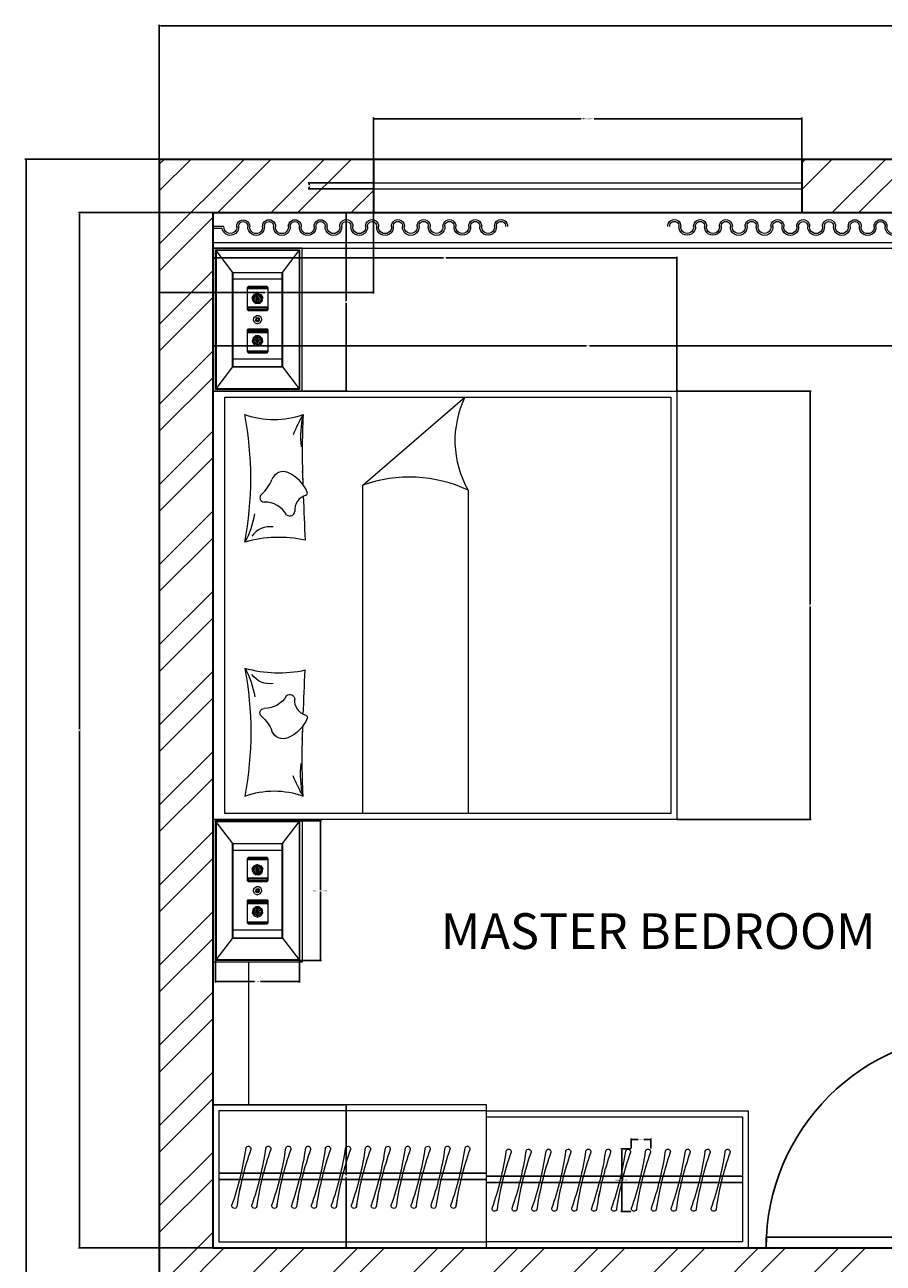
# Model space of a CAD drawing. Units: inches. Extents: x 3449 to 3843, y 1566 to 2054.
# Tile 6 of 8: x 3449 to 3594, y 1846 to 2054. Entities that reach past the tile are written whole.
import ezdxf

# ---------------------------------------------------------------- set-up
doc = ezdxf.new("R2010")
doc.units = ezdxf.units.IN
for name, color, linetype, lineweight in [('A-ANNO-DIMS', 2, 'Continuous', 18), ('A-AREA-IDEN', 7, 'Continuous', 25), ('A-DOOR', 4, 'Continuous', 25), ('A-FLOR-CASE', 7, 'Continuous', 20), ('A-FURN-DRAP', 32, 'Continuous', 13), ('A-GLAZ', 5, 'Continuous', 18), ('A-WALL', 7, 'Continuous', 35), ('A-WALL-PATT', 251, 'Continuous', 13), ('furn', 7, 'Continuous', 18)]:
    doc.layers.add(name, color=color, linetype=linetype, lineweight=lineweight)
doc.styles.get("Standard").update_dxf_attribs({"font": 'arial.ttf'})
doc.dimstyles.get("Standard").update_dxf_attribs({"dimtxt": 0.18, "dimasz": 0.18, "dimexe": 0.18, "dimexo": 0.0625, "dimgap": 0.09, "dimtad": 0, "dimtih": 1, "dimtoh": 1, "dimdec": 4, "dimzin": 0, "dimdsep": 46, "dimtxsty": 'Standard', "dimcen": 0.09, "dimadec": 0, "dimazin": 0, "dimtfac": 1, "dimtdec": 4, "dimtofl": 0, "dimtmove": 0, "dimatfit": 3, "dimfxl": 1, "dimtolj": 1, "dimtzin": 0, "dimarcsym": 0})

# ---------------------------------------------------------------- blocks, each defined once
blk = doc.blocks.new('*U5')
for p, q in [((0, 0), (0, -6)), ((36, 0), (36, -6))]:
    blk.add_line(p, q)
blk.add_lwpolyline([(0, 0), (0, 36), (1.75, 36), (1.75, 0)], close=True)
blk.add_arc((0, 0), 36, 0, 90)
blk = doc.blocks.new('12PLMP48')
for p, q in [((-4.94, 8.22), (-5, 8.31)), ((-5, 8.31), (5, 8.31)), ((-5, -8.31), (-5, 8.31)), ((-2.96, 5.62), (-4.94, 8.22)), ((4.94, 8.22), (-4.94, 8.22)), ((-4.94, 8.22), (-4.94, -8.22)), ((2.96, 5.62), (4.94, 8.22)), ((5, 8.31), (4.94, 8.22)), ((4.94, 8.22), (4.94, -8.22)), ((5, 8.31), (5, -8.31)), ((-2.94, 5.59), (-3, 5.62)), ((-3, 5.62), (3, 5.62)), ((-3, -5.63), (-3, 5.62)), ((2.94, 5.59), (-2.94, 5.59)), ((-2.94, 5.59), (-2.94, -5.59)), ((2.94, 4.81), (-2.94, 4.81)), ((3, 5.62), (2.94, 5.59)), ((2.94, -5.59), (2.94, 5.59)), ((3, -5.63), (3, 5.62)), ((-1.13, 3.94), (-1.25, 3.81)), ((-1.13, 3.84), (-1.25, 3.72)), ((-1.25, 3.81), (-1.25, 1.22)), ((-1.25, 3.72), (1.25, 3.72)), ((1.13, 3.94), (-1.13, 3.94)), ((-1.13, 3.84), (-1.13, 3.94)), ((1.13, 3.84), (-1.13, 3.84)), ((-0.62, 2.61), (-0.4, 2.98)), ((0, 3.12), (-0.4, 2.98)), ((-0.4, 2.98), (-0.32, 2.88)), ((0, 3), (-0.32, 2.88)), ((0, 2.5), (0, 3.12)), ((0, 3.12), (0.4, 2.98)), ((0.32, 2.88), (0, 3)), ((0.32, 2.88), (0.4, 2.98)), ((0.4, 2.98), (0.62, 2.61)), ((1.25, 3.81), (1.13, 3.94)), ((1.13, 3.84), (1.13, 3.94)), ((1.25, 3.72), (1.13, 3.84)), ((1.25, 1.22), (1.25, 3.81)), ((-1.13, 1.41), (-1.25, 1.53)), ((-1.25, 1.53), (1.25, 1.53)), ((0, 2.5), (-0.62, 2.61)), ((-0.54, 2.19), (-0.62, 2.61)), ((-0.38, 2.28), (-0.54, 2.19)), ((-0.54, 2.19), (-0.21, 1.91)), ((-0.32, 2.88), (-0.49, 2.59)), ((-0.49, 2.59), (-0.43, 2.25)), ((-0.43, 2.58), (-0.28, 2.83)), ((-0.38, 2.28), (-0.43, 2.58)), ((-0.43, 2.25), (-0.17, 2.03)), ((0, 2.5), (-0.38, 2.28)), ((-0.15, 2.09), (-0.38, 2.28)), ((-0.32, 2.88), (-0.32, 2.88)), ((-0.32, 2.88), (-0.28, 2.83)), ((-0.28, 2.83), (0, 2.94)), ((-0.28, 2.83), (0, 2.5)), ((-0.21, 1.91), (0, 2.5)), ((0.21, 1.91), (-0.21, 1.91)), ((-0.17, 2.03), (0.17, 2.03)), ((0.15, 2.09), (-0.15, 2.09)), ((-0.08, 2.6), (-0.12, 2.52)), ((-0.12, 2.52), (-0.11, 2.44)), ((-0.11, 2.44), (-0.04, 2.38)), ((0, 2.62), (-0.08, 2.6)), ((-0.04, 2.38), (0.04, 2.38)), ((0, 2.94), (0.28, 2.83)), ((0, 2.5), (0.32, 2.88)), ((0.08, 2.6), (0, 2.62)), ((0.62, 2.61), (0, 2.5)), ((0.54, 2.19), (0, 2.5)), ((0, 2.5), (0.21, 1.91)), ((0.04, 2.38), (0.11, 2.44)), ((0.12, 2.52), (0.08, 2.6)), ((0.11, 2.44), (0.12, 2.52)), ((0.38, 2.28), (0.15, 2.09)), ((0.17, 2.03), (0.43, 2.25)), ((0.21, 1.91), (0.54, 2.19)), ((0.28, 2.83), (0.43, 2.58)), ((0.49, 2.59), (0.32, 2.88)), ((0.32, 2.88), (0.32, 2.88)), ((0.43, 2.58), (0.38, 2.28)), ((0.43, 2.25), (0.49, 2.59)), ((0.54, 2.19), (0.62, 2.61)), ((1.25, 1.53), (1.13, 1.41)), ((-1.13, 1.25), (-1.25, 1.37)), ((-1.25, 1.22), (-1.13, 1.09)), ((1.13, 1.41), (-1.13, 1.41)), ((-1.13, 1.41), (-1.13, 1.09)), ((-1.13, 1.25), (1.13, 1.25)), ((-1.13, 1.09), (1.13, 1.09)), ((-0.49, -0.09), (-0.43, 0.25)), ((-0.43, 0.25), (-0.17, 0.47)), ((-0.22, 0.12), (-0.25, -0.04)), ((-0.09, 0.23), (-0.22, 0.12)), ((0.17, 0.47), (-0.17, 0.47)), ((-0.12, -0.12), (-0.12, 0.12)), ((-0.12, 0.12), (0.12, 0.12)), ((-0.09, 0.23), (0.09, 0.23)), ((0.22, 0.12), (0.09, 0.23)), ((0.12, 0.12), (0.12, -0.12)), ((0.43, 0.25), (0.17, 0.47)), ((0.25, -0.04), (0.22, 0.12)), ((0.43, 0.25), (0.49, -0.09)), ((1.13, 1.09), (1.13, 1.41)), ((1.13, 1.25), (1.25, 1.37)), ((1.13, 1.09), (1.25, 1.22)), ((-1.25, -1.22), (-1.13, -1.09)), ((-1.25, -1.22), (-1.25, -3.81)), ((-1.13, -1.25), (-1.25, -1.38)), ((-1.13, -1.41), (-1.25, -1.53)), ((-1.13, -1.41), (-1.13, -1.09)), ((-1.13, -1.09), (1.13, -1.09)), ((1.13, -1.25), (-1.13, -1.25)), ((1.13, -1.41), (-1.13, -1.41)), ((-0.32, -0.38), (-0.49, -0.09)), ((-0.32, -0.38), (0, -0.5)), ((-0.16, -0.19), (-0.25, -0.04)), ((0, -0.25), (-0.16, -0.19)), ((0.12, -0.12), (-0.12, -0.12)), ((0.16, -0.19), (0, -0.25)), ((0.32, -0.38), (0, -0.5)), ((0.16, -0.19), (0.25, -0.04)), ((0.32, -0.38), (0.49, -0.09)), ((1.13, -1.41), (1.13, -1.09)), ((1.13, -1.09), (1.25, -1.22)), ((1.25, -1.38), (1.13, -1.25)), ((1.25, -1.53), (1.13, -1.41)), ((1.25, -3.81), (1.25, -1.22)), ((-1.25, -1.53), (1.25, -1.53)), ((-0.54, -2.19), (-0.62, -2.61)), ((0, -2.5), (-0.62, -2.61)), ((-0.62, -2.61), (-0.4, -2.98)), ((-0.21, -1.91), (-0.54, -2.19)), ((-0.54, -2.19), (0, -2.5)), ((-0.49, -2.59), (-0.43, -2.25)), ((-0.32, -2.88), (-0.49, -2.59)), ((-0.43, -2.25), (-0.17, -2.03)), ((-0.43, -2.58), (-0.38, -2.28)), ((-0.28, -2.84), (-0.43, -2.58)), ((-0.4, -2.98), (-0.32, -2.88)), ((-0.38, -2.28), (-0.15, -2.09)), ((-0.32, -2.88), (-0.28, -2.84)), ((0, -3), (-0.32, -2.88)), ((-0.28, -2.84), (-0.08, -2.6)), ((0, -2.94), (-0.28, -2.84)), ((0.21, -1.91), (-0.21, -1.91)), ((0, -2.5), (-0.21, -1.91)), ((-0.17, -2.03), (0.17, -2.03)), ((-0.15, -2.09), (0.15, -2.09)), ((-0.11, -2.44), (-0.12, -2.52)), ((-0.12, -2.52), (-0.08, -2.6)), ((-0.04, -2.38), (-0.11, -2.44)), ((-0.08, -2.6), (0, -2.5)), ((-0.08, -2.6), (0, -2.63)), ((0.04, -2.38), (-0.04, -2.38)), ((0, -2.5), (0.21, -1.91)), ((0.11, -2.44), (0, -2.5)), ((0, -3.13), (0, -2.5)), ((0, -2.5), (0.4, -2.98)), ((0.62, -2.61), (0, -2.5)), ((0, -2.63), (0.08, -2.6)), ((0.28, -2.84), (0, -2.94)), ((0.32, -2.88), (0, -3)), ((0.11, -2.44), (0.04, -2.38)), ((0.08, -2.6), (0.12, -2.52)), ((0.38, -2.28), (0.11, -2.44)), ((0.12, -2.52), (0.11, -2.44)), ((0.15, -2.09), (0.38, -2.28)), ((0.17, -2.03), (0.43, -2.25)), ((0.21, -1.91), (0.54, -2.19)), ((0.43, -2.58), (0.28, -2.84)), ((0.49, -2.59), (0.32, -2.88)), ((0.54, -2.19), (0.38, -2.28)), ((0.38, -2.28), (0.43, -2.58)), ((0.4, -2.98), (0.62, -2.61)), ((0.43, -2.25), (0.49, -2.59)), ((0.62, -2.61), (0.54, -2.19)), ((-1.13, -3.84), (-1.25, -3.72)), ((-1.25, -3.72), (1.25, -3.72)), ((-1.25, -3.81), (-1.13, -3.94)), ((-1.13, -3.94), (-1.13, -3.84)), ((1.13, -3.84), (-1.13, -3.84)), ((-1.13, -3.94), (1.13, -3.94)), ((-0.4, -2.98), (0, -3.13)), ((0, -3.13), (0.4, -2.98)), ((1.25, -3.72), (1.13, -3.84)), ((1.13, -3.94), (1.25, -3.81)), ((1.13, -3.94), (1.13, -3.84)), ((-4.94, -8.22), (-2.96, -5.63)), ((-2.94, -5.59), (-3, -5.63)), ((-3, -5.63), (3, -5.63)), ((2.94, -4.69), (-2.94, -4.69)), ((-2.94, -5.59), (2.94, -5.59)), ((3, -5.63), (2.94, -5.59)), ((2.96, -5.63), (4.94, -8.22)), ((-4.94, -8.22), (-5, -8.31)), ((5, -8.31), (-5, -8.31)), ((4.94, -8.22), (-4.94, -8.22)), ((4.94, -8.22), (5, -8.31))]:
    blk.add_line(p, q)
blk = doc.blocks.new('PILLOW-BED')
for centre, radius, start, end in [((-58.04, 10.73), 59.02, 349.525, 10.475), ((4.89, 35.06), 14.45, 250.2291, 289.7709), ((27.88, 10.54), 21.14, 148.9025, 159.1397), ((25.99, 17.7), 16.64, 166.9326, 185.8487), ((149.01, 15.02), 139.38, 177.3527, 182.1874), ((370.18, 15.14), 360.55, 180.0403, 180.0472), ((-1.15, 12.67), 6.07, 310.2522, 339.5725), ((6.42, 9.85), 2, 66.6818, 159.5725), ((4.74, 5.96), 6.24, 23.0209, 66.6818), ((56.2, 13.08), 46.57, 181.419, 184.1998), ((10.15, 8.25), 0.362, 287.5153, 24.7447), ((3.25, 7.48), 0.73, 130.2522, 270.4936), ((3.29, 2.5), 4.25, 29.3034, 90.4936), ((10.95, 5.41), 2.59, 105.4046, 185.5925), ((370.18, 19.17), 360.55, 181.8172, 182.9967), ((-12.31, 6.94), 14.13, 330.5975, 351.1793), ((7.53, 5.25), 0.85, 231.2945, 354.0462), ((4.17, -1.03), 3.63, 80.7217, 145.7354), ((5.68, -19.42), 20.23, 77.3054, 106.2929)]:
    blk.add_arc(centre, radius, start, end)
blk = doc.blocks.new('DRAPERY-PANEL')
for p, q in [((1.19, 47.95), (1.19, 49.52)), ((1.5, 47.66), (1.5, 49.52))]:
    blk.add_line(p, q)
for centre, radius, start, end in [((1.42, 46.57), 1.4, 99.481, 274.2422), ((1.42, 46.57), 1.09, 85.7578, 274.2422), ((1.55, 44.41), 1.09, 265.7578, 94.2422), ((1.55, 44.41), 0.776, 265.7578, 94.2422), ((1.4, 42.24), 1.4, 85.7578, 274.2422), ((1.4, 42.24), 1.09, 85.7578, 274.2422), ((1.56, 40.07), 1.09, 265.7578, 94.2422), ((1.56, 40.07), 0.776, 265.7578, 94.2422), ((1.4, 37.91), 1.4, 85.7578, 274.2422), ((1.4, 37.91), 1.09, 85.7578, 274.2422), ((1.56, 35.74), 1.09, 265.7578, 94.2422), ((1.56, 35.74), 0.776, 265.7578, 94.2422), ((1.4, 33.58), 1.4, 85.7578, 274.2422), ((1.4, 33.58), 1.09, 85.7578, 274.2422), ((1.56, 31.41), 1.09, 265.7578, 94.2422), ((1.56, 31.41), 0.776, 265.7578, 94.2422), ((1.41, 29.24), 1.4, 85.7578, 274.2422), ((1.41, 29.24), 1.09, 85.7578, 274.2422), ((1.57, 27.08), 1.09, 265.7578, 94.2422), ((1.57, 27.08), 0.776, 265.7578, 94.2422), ((1.41, 24.91), 1.4, 85.7578, 274.2422), ((1.41, 24.91), 1.09, 85.7578, 274.2422), ((1.57, 22.74), 1.09, 265.7578, 94.2422), ((1.57, 22.74), 0.776, 265.7578, 94.2422), ((1.41, 20.58), 1.4, 85.7578, 274.2422), ((1.41, 20.58), 1.09, 85.7578, 274.2422), ((1.58, 18.41), 1.09, 265.7578, 94.2422), ((1.58, 18.41), 0.776, 265.7578, 94.2422), ((1.42, 16.25), 1.4, 85.7578, 274.2422), ((1.42, 16.25), 1.09, 85.7578, 274.2422), ((1.58, 14.08), 1.09, 265.7578, 94.2422), ((1.58, 14.08), 0.776, 265.7578, 94.2422), ((1.42, 11.91), 1.4, 85.7578, 274.2422), ((1.42, 11.91), 1.09, 85.7578, 274.2422), ((1.58, 9.75), 1.09, 265.7578, 94.2422), ((1.58, 9.75), 0.776, 265.7578, 94.2422), ((1.43, 7.58), 1.4, 85.7578, 274.2422), ((1.43, 7.58), 1.09, 85.7578, 274.2422), ((1.59, 5.42), 1.09, 265.7578, 94.2422), ((1.43, 3.25), 1.4, 85.7578, 274.2422), ((1.43, 3.25), 1.09, 85.7578, 274.2422), ((1.59, 5.42), 0.776, 265.7578, 94.2422), ((1.59, 1.08), 1.09, 265.7578, 94.2422), ((1.59, 1.08), 0.776, 265.7578, 94.2422)]:
    blk.add_arc(centre, radius, start, end)
blk = doc.blocks.new('DRAPERY-PANEL-CAPPED')
for p, q in [((1.19, 1.57), (1.19, 0)), ((1.19, 0), (1.5, 0)), ((1.5, 1.86), (1.5, 0))]:
    blk.add_line(p, q)
for centre, radius, start, end in [((1.59, 48.44), 1.09, 265.7578, 94.2422), ((1.59, 48.44), 0.776, 265.7578, 94.2422), ((1.43, 46.27), 1.4, 85.7578, 274.2422), ((1.43, 46.27), 1.09, 85.7578, 274.2422), ((1.59, 44.1), 1.09, 265.7578, 94.2422), ((1.59, 44.1), 0.776, 265.7578, 94.2422), ((1.43, 41.94), 1.4, 85.7578, 274.2422), ((1.43, 41.94), 1.09, 85.7578, 274.2422), ((1.58, 39.77), 1.09, 265.7578, 94.2422), ((1.58, 39.77), 0.776, 265.7578, 94.2422), ((1.42, 37.6), 1.4, 85.7578, 274.2422), ((1.42, 37.6), 1.09, 85.7578, 274.2422), ((1.58, 35.44), 1.09, 265.7578, 94.2422), ((1.58, 35.44), 0.776, 265.7578, 94.2422), ((1.42, 33.27), 1.4, 85.7578, 274.2422), ((1.42, 33.27), 1.09, 85.7578, 274.2422), ((1.58, 31.11), 1.09, 265.7578, 94.2422), ((1.58, 31.11), 0.776, 265.7578, 94.2422), ((1.41, 28.94), 1.4, 85.7578, 274.2422), ((1.41, 28.94), 1.09, 85.7578, 274.2422), ((1.57, 26.77), 1.09, 265.7578, 94.2422), ((1.57, 26.77), 0.776, 265.7578, 94.2422), ((1.41, 24.61), 1.4, 85.7578, 274.2422), ((1.41, 24.61), 1.09, 85.7578, 274.2422), ((1.57, 22.44), 1.09, 265.7578, 94.2422), ((1.57, 22.44), 0.776, 265.7578, 94.2422), ((1.41, 20.28), 1.4, 85.7578, 274.2422), ((1.41, 20.28), 1.09, 85.7578, 274.2422), ((1.56, 18.11), 1.09, 265.7578, 94.2422), ((1.56, 18.11), 0.776, 265.7578, 94.2422), ((1.4, 15.94), 1.4, 85.7578, 274.2422), ((1.4, 15.94), 1.09, 85.7578, 274.2422), ((1.56, 13.78), 1.09, 265.7578, 94.2422), ((1.4, 11.61), 1.4, 85.7578, 274.2422), ((1.4, 11.61), 1.09, 85.7578, 274.2422), ((1.56, 13.78), 0.776, 265.7578, 94.2422), ((1.56, 9.45), 1.09, 265.7578, 94.2422), ((1.4, 7.28), 1.4, 85.7578, 274.2422), ((1.4, 7.28), 1.09, 85.7578, 274.2422), ((1.56, 9.45), 0.776, 265.7578, 94.2422), ((1.42, 2.95), 1.4, 85.7578, 260.519), ((1.55, 5.11), 1.09, 265.7578, 94.2422), ((1.55, 5.11), 0.776, 265.7578, 94.2422), ((1.42, 2.95), 1.09, 85.7578, 274.2422)]:
    blk.add_arc(centre, radius, start, end)
blk = doc.blocks.new('WARDROBE-HANGER-A')
at = {"transparency": 33554687}
blk.add_lwpolyline([(2.38, 10.13, -1), (3.19, 9.92, 0.050016), (0.83, 0.32, -1), (0.01, 0.52, 0.050016)], format="xyb", close=True, dxfattribs=at)
blk.add_arc((49.86, -6.67), 49.53, 160.4279, 171.8811, dxfattribs=at)
blk = doc.blocks.new('WARDROBE-HANGER-B')
at = {"transparency": 33554687}
blk.add_lwpolyline([(2.37, 10.13, -1), (3.19, 9.92, 0.050016), (0.83, 0.32, -1), (0.01, 0.52, 0.050016)], format="xyb", close=True, dxfattribs=at)
blk.add_arc((49.86, -6.67), 49.53, 160.4279, 171.8811, dxfattribs=at)
blk = doc.blocks.new('GLAZING-72')
for p, q in [((0, 1), (72, 1)), ((0, 0), (72, 0))]:
    blk.add_line(p, q)
blk = doc.blocks.new('*D36')
at = {"layer": 'A-ANNO-DIMS', "color": 0, "lineweight": -2, "transparency": 16777216}
for p, q in [((3551.34, 1865.22), (3549.65, 1865.22)), ((3549.83, 1865.04), (3549.83, 1860.14)), ((3549.83, 1854.87), (3549.83, 1859.77)), ((3551.34, 1854.69), (3549.65, 1854.69))]:
    blk.add_line(p, q, dxfattribs=at)
at = {"layer": 'A-ANNO-DIMS', "color": 0, "transparency": 16777216}
for points in [[(3549.8, 1865.04), (3549.86, 1865.04), (3549.83, 1865.22)], [(3549.8, 1854.87), (3549.86, 1854.87), (3549.83, 1854.69)]]:
    blk.add_solid(points, dxfattribs=at)
at = {"layer": 'Defpoints', "color": 0, "transparency": 16777216}
for p in [(3549.83, 1865.22), (3551.41, 1865.22), (3551.41, 1854.69)]:
    blk.add_point(p, dxfattribs=at)
at = {"layer": 'A-ANNO-DIMS', "color": 0, "transparency": 16777216, "insert": (3549.83, 1859.96), "char_height": 0.18, "attachment_point": 5}
blk.add_mtext('\\A1;HANGER B 11 TYP.', dxfattribs=at)
blk = doc.blocks.new('*D37')
at = {"layer": 'A-ANNO-DIMS', "color": 0, "lineweight": -2, "transparency": 16777216}
for p, q in [((3551.41, 1865.29), (3551.41, 1866.99)), ((3551.59, 1866.81), (3552.6, 1866.81)), ((3554.52, 1866.81), (3553.51, 1866.81)), ((3554.7, 1865.29), (3554.7, 1866.99))]:
    blk.add_line(p, q, dxfattribs=at)
at = {"layer": 'A-ANNO-DIMS', "color": 0, "transparency": 16777216}
for points in [[(3551.59, 1866.84), (3551.59, 1866.78), (3551.41, 1866.81)], [(3554.52, 1866.84), (3554.52, 1866.78), (3554.7, 1866.81)]]:
    blk.add_solid(points, dxfattribs=at)
at = {"layer": 'Defpoints', "color": 0, "transparency": 16777216}
for p in [(3554.7, 1866.81), (3551.41, 1865.22), (3554.7, 1865.22)]:
    blk.add_point(p, dxfattribs=at)
at = {"layer": 'A-ANNO-DIMS', "color": 0, "transparency": 16777216, "insert": (3553.05, 1866.81), "char_height": 0.18, "attachment_point": 5}
blk.add_mtext('\\A1;3 TYP.', dxfattribs=at)
blk = doc.blocks.new('*D44')
at = {"layer": 'A-ANNO-DIMS', "color": 0, "lineweight": -2, "transparency": 16777216}
for p, q in [((3495.73, 1920.36), (3499.36, 1920.36)), ((3499.18, 1920.18), (3499.18, 1908.8)), ((3499.18, 1897.07), (3499.18, 1908.44)), ((3495.73, 1896.89), (3499.36, 1896.89))]:
    blk.add_line(p, q, dxfattribs=at)
at = {"layer": 'A-ANNO-DIMS', "color": 0, "transparency": 16777216}
for points in [[(3499.15, 1920.18), (3499.21, 1920.18), (3499.18, 1920.36)], [(3499.15, 1897.07), (3499.21, 1897.07), (3499.18, 1896.89)]]:
    blk.add_solid(points, dxfattribs=at)
at = {"layer": 'Defpoints', "color": 0, "transparency": 16777216}
for p in [(3495.66, 1920.36), (3499.18, 1920.36), (3495.66, 1896.89)]:
    blk.add_point(p, dxfattribs=at)
at = {"layer": 'A-ANNO-DIMS', "color": 0, "transparency": 16777216, "insert": (3499.18, 1908.62), "char_height": 0.18, "attachment_point": 5}
blk.add_mtext('\\A1;NIGHTSTAND 23 TYP.', dxfattribs=at)
blk = doc.blocks.new('*D45')
at = {"layer": 'A-ANNO-DIMS', "color": 0, "lineweight": -2, "transparency": 16777216}
for p, q in [((3481.55, 1896.82), (3481.55, 1893.18)), ((3495.66, 1896.82), (3495.66, 1893.18)), ((3481.73, 1893.36), (3488.09, 1893.36)), ((3495.48, 1893.36), (3489.12, 1893.36))]:
    blk.add_line(p, q, dxfattribs=at)
at = {"layer": 'A-ANNO-DIMS', "color": 0, "transparency": 16777216}
for points in [[(3481.73, 1893.39), (3481.73, 1893.33), (3481.55, 1893.36)], [(3495.48, 1893.39), (3495.48, 1893.33), (3495.66, 1893.36)]]:
    blk.add_solid(points, dxfattribs=at)
at = {"layer": 'Defpoints', "color": 0, "transparency": 16777216}
for p in [(3481.55, 1896.89), (3495.66, 1896.89), (3495.66, 1893.36)]:
    blk.add_point(p, dxfattribs=at)
at = {"layer": 'A-ANNO-DIMS', "color": 0, "transparency": 16777216, "insert": (3488.6, 1893.36), "char_height": 0.18, "attachment_point": 5}
blk.add_mtext('\\A1;14 TYP.', dxfattribs=at)
blk = doc.blocks.new('*D60')
at = {"layer": 'A-ANNO-DIMS', "color": 0, "lineweight": -2, "transparency": 16777216}
for p, q in [((3508.09, 2027.68), (3508.09, 2038.59)), ((3508.27, 2038.41), (3542.97, 2038.41)), ((3579.91, 2038.41), (3545.21, 2038.41)), ((3580.09, 2027.68), (3580.09, 2038.59))]:
    blk.add_line(p, q, dxfattribs=at)
at = {"layer": 'A-ANNO-DIMS', "color": 0, "transparency": 16777216}
for points in [[(3508.27, 2038.44), (3508.27, 2038.38), (3508.09, 2038.41)], [(3579.91, 2038.44), (3579.91, 2038.38), (3580.09, 2038.41)]]:
    blk.add_solid(points, dxfattribs=at)
at = {"layer": 'Defpoints', "color": 0, "transparency": 16777216}
for p in [(3580.09, 2038.41), (3508.09, 2027.61), (3580.09, 2027.61)]:
    blk.add_point(p, dxfattribs=at)
at = {"layer": 'A-ANNO-DIMS', "color": 0, "transparency": 16777216, "insert": (3544.09, 2038.41), "char_height": 0.18, "attachment_point": 5}
blk.add_mtext('\\A1;WINDOW 72 TYP.', dxfattribs=at)
blk = doc.blocks.new('*D61')
at = {"layer": 'A-ANNO-DIMS', "color": 0, "lineweight": -2, "transparency": 16777216}
for p, q in [((3508.03, 2027.61), (3497.11, 2027.61)), ((3508.03, 2026.61), (3497.11, 2026.61)), ((3497.29, 2027.43), (3497.29, 2027.29)), ((3497.29, 2026.79), (3497.29, 2026.93))]:
    blk.add_line(p, q, dxfattribs=at)
at = {"layer": 'A-ANNO-DIMS', "color": 0, "transparency": 16777216}
for points in [[(3497.26, 2027.43), (3497.32, 2027.43), (3497.29, 2027.61)], [(3497.26, 2026.79), (3497.32, 2026.79), (3497.29, 2026.61)]]:
    blk.add_solid(points, dxfattribs=at)
at = {"layer": 'Defpoints', "color": 0, "transparency": 16777216}
for p in [(3497.29, 2027.61), (3508.09, 2027.61), (3508.09, 2026.61)]:
    blk.add_point(p, dxfattribs=at)
at = {"layer": 'A-ANNO-DIMS', "color": 0, "transparency": 16777216, "insert": (3497.29, 2027.11), "char_height": 0.18, "attachment_point": 5}
blk.add_mtext('\\A1;1 TYP.', dxfattribs=at)
blk = doc.blocks.new('*D76')
at = {"layer": 'A-ANNO-DIMS', "color": 0, "lineweight": -2, "transparency": 16777216}
for p, q in [((3472.09, 2031.68), (3472.09, 2054.19)), ((3472.27, 2054.01), (3645.8, 2054.01)), ((3819.91, 2054.01), (3646.38, 2054.01)), ((3820.09, 1986.68), (3820.09, 2054.19))]:
    blk.add_line(p, q, dxfattribs=at)
at = {"layer": 'A-ANNO-DIMS', "color": 0, "transparency": 16777216}
for points in [[(3472.27, 2054.04), (3472.27, 2053.98), (3472.09, 2054.01)], [(3819.91, 2054.04), (3819.91, 2053.98), (3820.09, 2054.01)]]:
    blk.add_solid(points, dxfattribs=at)
at = {"layer": 'Defpoints', "color": 0, "transparency": 16777216}
for p in [(3820.09, 2054.01), (3472.09, 2031.61), (3820.09, 1986.61)]:
    blk.add_point(p, dxfattribs=at)
at = {"layer": 'A-ANNO-DIMS', "color": 0, "transparency": 16777216, "insert": (3646.09, 2054.01), "char_height": 0.18, "attachment_point": 5}
blk.add_mtext('\\A1;348', dxfattribs=at)
blk = doc.blocks.new('*D77')
at = {"layer": 'A-ANNO-DIMS', "color": 0, "lineweight": -2, "transparency": 16777216}
for p, q in [((3472.03, 2031.61), (3449.51, 2031.61)), ((3449.69, 2031.43), (3449.69, 1810.3)), ((3449.69, 1588.79), (3449.69, 1809.93)), ((3481.03, 1588.61), (3449.51, 1588.61))]:
    blk.add_line(p, q, dxfattribs=at)
at = {"layer": 'A-ANNO-DIMS', "color": 0, "transparency": 16777216}
for points in [[(3449.66, 2031.43), (3449.72, 2031.43), (3449.69, 2031.61)], [(3449.66, 1588.79), (3449.72, 1588.79), (3449.69, 1588.61)]]:
    blk.add_solid(points, dxfattribs=at)
at = {"layer": 'Defpoints', "color": 0, "transparency": 16777216}
for p in [(3449.69, 2031.61), (3472.09, 2031.61), (3481.09, 1588.61)]:
    blk.add_point(p, dxfattribs=at)
at = {"layer": 'A-ANNO-DIMS', "color": 0, "transparency": 16777216, "insert": (3449.69, 1810.11), "char_height": 0.18, "attachment_point": 5}
blk.add_mtext('\\A1;443', dxfattribs=at)
blk = doc.blocks.new('*D80')
at = {"layer": 'A-ANNO-DIMS', "color": 0, "lineweight": -2, "transparency": 16777216}
for p, q in [((3472.09, 2031.55), (3472.09, 2009.03)), ((3508.09, 2031.55), (3508.09, 2009.03)), ((3472.27, 2009.21), (3489.87, 2009.21)), ((3507.91, 2009.21), (3490.31, 2009.21))]:
    blk.add_line(p, q, dxfattribs=at)
at = {"layer": 'A-ANNO-DIMS', "color": 0, "transparency": 16777216}
for points in [[(3472.27, 2009.24), (3472.27, 2009.18), (3472.09, 2009.21)], [(3507.91, 2009.24), (3507.91, 2009.18), (3508.09, 2009.21)]]:
    blk.add_solid(points, dxfattribs=at)
at = {"layer": 'Defpoints', "color": 0, "transparency": 16777216}
for p in [(3472.09, 2031.61), (3508.09, 2031.61), (3472.09, 2009.21)]:
    blk.add_point(p, dxfattribs=at)
at = {"layer": 'A-ANNO-DIMS', "color": 0, "transparency": 16777216, "insert": (3490.09, 2009.21), "char_height": 0.18, "attachment_point": 5}
blk.add_mtext('\\A1;36', dxfattribs=at)
blk = doc.blocks.new('*D81')
at = {"layer": 'A-ANNO-DIMS', "color": 0, "lineweight": -2, "transparency": 16777216}
for p, q in [((3481.03, 2022.61), (3458.51, 2022.61)), ((3458.69, 2022.43), (3458.69, 1935.79)), ((3458.69, 1848.79), (3458.69, 1935.43)), ((3481.03, 1848.61), (3458.51, 1848.61))]:
    blk.add_line(p, q, dxfattribs=at)
at = {"layer": 'A-ANNO-DIMS', "color": 0, "transparency": 16777216}
for points in [[(3458.66, 2022.43), (3458.72, 2022.43), (3458.69, 2022.61)], [(3458.66, 1848.79), (3458.72, 1848.79), (3458.69, 1848.61)]]:
    blk.add_solid(points, dxfattribs=at)
at = {"layer": 'Defpoints', "color": 0, "transparency": 16777216}
for p in [(3458.69, 2022.61), (3481.09, 2022.61), (3481.09, 1848.61)]:
    blk.add_point(p, dxfattribs=at)
at = {"layer": 'A-ANNO-DIMS', "color": 0, "transparency": 16777216, "insert": (3458.69, 1935.61), "char_height": 0.18, "attachment_point": 5}
blk.add_mtext('\\A1;174', dxfattribs=at)
blk = doc.blocks.new('*D82')
at = {"layer": 'A-ANNO-DIMS', "color": 0, "lineweight": -2, "transparency": 16777216}
for p, q in [((3481.09, 2022.55), (3481.09, 2000.03)), ((3607.09, 2022.55), (3607.09, 2000.03)), ((3481.27, 2000.21), (3543.81, 2000.21)), ((3606.91, 2000.21), (3544.37, 2000.21))]:
    blk.add_line(p, q, dxfattribs=at)
at = {"layer": 'A-ANNO-DIMS', "color": 0, "transparency": 16777216}
for points in [[(3481.27, 2000.24), (3481.27, 2000.18), (3481.09, 2000.21)], [(3606.91, 2000.24), (3606.91, 2000.18), (3607.09, 2000.21)]]:
    blk.add_solid(points, dxfattribs=at)
at = {"layer": 'Defpoints', "color": 0, "transparency": 16777216}
for p in [(3481.09, 2022.61), (3607.09, 2022.61), (3481.09, 2000.21)]:
    blk.add_point(p, dxfattribs=at)
at = {"layer": 'A-ANNO-DIMS', "color": 0, "transparency": 16777216, "insert": (3544.09, 2000.21), "char_height": 0.18, "attachment_point": 5}
blk.add_mtext('\\A1;126', dxfattribs=at)
blk = doc.blocks.new('*D103')
at = {"layer": 'A-ANNO-DIMS', "color": 0, "lineweight": -2, "transparency": 16777216}
for p, q in [((3481.09, 1992.68), (3481.09, 2015.19)), ((3481.27, 2015.01), (3519.87, 2015.01)), ((3558.91, 2015.01), (3520.31, 2015.01)), ((3559.09, 1992.68), (3559.09, 2015.19))]:
    blk.add_line(p, q, dxfattribs=at)
at = {"layer": 'A-ANNO-DIMS', "color": 0, "transparency": 16777216}
for points in [[(3481.27, 2015.04), (3481.27, 2014.98), (3481.09, 2015.01)], [(3558.91, 2015.04), (3558.91, 2014.98), (3559.09, 2015.01)]]:
    blk.add_solid(points, dxfattribs=at)
at = {"layer": 'Defpoints', "color": 0, "transparency": 16777216}
for p in [(3559.09, 2015.01), (3481.09, 1992.61), (3559.09, 1992.61)]:
    blk.add_point(p, dxfattribs=at)
at = {"layer": 'A-ANNO-DIMS', "color": 0, "transparency": 16777216, "insert": (3520.09, 2015.01), "char_height": 0.18, "attachment_point": 5}
blk.add_mtext('\\A1;78', dxfattribs=at)
blk = doc.blocks.new('*D104')
at = {"layer": 'A-ANNO-DIMS', "color": 0, "lineweight": -2, "transparency": 16777216}
for p, q in [((3559.15, 1992.61), (3581.67, 1992.61)), ((3581.49, 1992.43), (3581.49, 1956.79)), ((3581.49, 1920.79), (3581.49, 1956.43)), ((3559.15, 1920.61), (3581.67, 1920.61))]:
    blk.add_line(p, q, dxfattribs=at)
at = {"layer": 'A-ANNO-DIMS', "color": 0, "transparency": 16777216}
for points in [[(3581.46, 1992.43), (3581.52, 1992.43), (3581.49, 1992.61)], [(3581.46, 1920.79), (3581.52, 1920.79), (3581.49, 1920.61)]]:
    blk.add_solid(points, dxfattribs=at)
at = {"layer": 'Defpoints', "color": 0, "transparency": 16777216}
for p in [(3559.09, 1992.61), (3559.09, 1920.61), (3581.49, 1920.61)]:
    blk.add_point(p, dxfattribs=at)
at = {"layer": 'A-ANNO-DIMS', "color": 0, "transparency": 16777216, "insert": (3581.49, 1956.61), "char_height": 0.18, "attachment_point": 5}
blk.add_mtext('\\A1;72', dxfattribs=at)
blk = doc.blocks.new('*D116')
at = {"layer": 'A-ANNO-DIMS', "color": 0, "lineweight": -2, "transparency": 16777216}
for p, q in [((3481.15, 2022.61), (3503.67, 2022.61)), ((3503.49, 2022.43), (3503.49, 2007.8)), ((3503.49, 1992.79), (3503.49, 2007.43)), ((3481.15, 1992.61), (3503.67, 1992.61))]:
    blk.add_line(p, q, dxfattribs=at)
at = {"layer": 'A-ANNO-DIMS', "color": 0, "transparency": 16777216}
for points in [[(3503.46, 2022.43), (3503.52, 2022.43), (3503.49, 2022.61)], [(3503.46, 1992.79), (3503.52, 1992.79), (3503.49, 1992.61)]]:
    blk.add_solid(points, dxfattribs=at)
at = {"layer": 'Defpoints', "color": 0, "transparency": 16777216}
for p in [(3481.09, 2022.61), (3481.09, 1992.61), (3503.49, 1992.61)]:
    blk.add_point(p, dxfattribs=at)
at = {"layer": 'A-ANNO-DIMS', "color": 0, "transparency": 16777216, "insert": (3503.49, 2007.61), "char_height": 0.18, "attachment_point": 5}
blk.add_mtext('\\A1;30', dxfattribs=at)
blk = doc.blocks.new('*D122')
at = {"layer": 'A-ANNO-DIMS', "color": 0, "lineweight": -2, "transparency": 16777216}
for p, q in [((3481.15, 1872.61), (3503.67, 1872.61)), ((3503.49, 1872.43), (3503.49, 1860.79)), ((3503.49, 1848.79), (3503.49, 1860.43)), ((3481.15, 1848.61), (3503.67, 1848.61))]:
    blk.add_line(p, q, dxfattribs=at)
at = {"layer": 'A-ANNO-DIMS', "color": 0, "transparency": 16777216}
for points in [[(3503.46, 1872.43), (3503.52, 1872.43), (3503.49, 1872.61)], [(3503.46, 1848.79), (3503.52, 1848.79), (3503.49, 1848.61)]]:
    blk.add_solid(points, dxfattribs=at)
at = {"layer": 'Defpoints', "color": 0, "transparency": 16777216}
for p in [(3481.09, 1872.61), (3481.09, 1848.61), (3503.49, 1848.61)]:
    blk.add_point(p, dxfattribs=at)
at = {"layer": 'A-ANNO-DIMS', "color": 0, "transparency": 16777216, "insert": (3503.49, 1860.61), "char_height": 0.18, "attachment_point": 5}
blk.add_mtext('\\A1;24', dxfattribs=at)

msp = doc.modelspace()

# ---------------------------------------------------------------- hatches: boundary and pattern name
at = {"layer": 'A-WALL-PATT'}
h = msp.add_hatch(dxfattribs=at)
h.set_pattern_fill('ANSI32', color=256)
edge = h.paths.add_edge_path()
edge.add_line((3481.088, 2022.6144), (3508.088, 2022.6144))
edge.add_line((3508.088, 2022.6144), (3508.088, 2031.6144))
edge.add_line((3508.088, 2031.6144), (3472.088, 2031.6144))
edge.add_line((3472.088, 2031.6144), (3472.088, 1779.6144))
edge.add_line((3472.088, 1779.6144), (3481.088, 1779.6144))
edge.add_line((3481.088, 1779.6144), (3481.088, 1839.6144))
edge.add_line((3481.088, 1839.6144), (3571.088, 1839.6144))
edge.add_line((3571.088, 1839.6144), (3571.088, 1824.3194))
edge.add_line((3571.088, 1824.3194), (3571.088, 1821.6144))
edge.add_line((3571.088, 1821.6144), (3580.088, 1821.6144))
edge.add_line((3580.088, 1821.6144), (3580.088, 1825.1908))
edge.add_ellipse((3580.1411, 1825.2442), major_axis=(0, 0.0754), ratio=0.99913951, start_angle=90, end_angle=135.183195, ccw=False)
edge.add_line((3580.0017, 1825.3196), (3580.0658, 1825.3196))
edge.add_line((3580.0658, 1825.3196), (3580.066, 1839.6365))
edge.add_line((3580.066, 1839.6365), (3616.088, 1839.6365))
edge.add_line((3616.088, 1839.6365), (3616.088, 1848.6144))
edge.add_line((3616.088, 1848.6144), (3610.088, 1848.6144))
edge.add_line((3610.088, 1848.6144), (3574.088, 1848.6144))
edge.add_line((3574.088, 1848.6144), (3481.088, 1848.6144))
edge.add_line((3481.088, 1848.6144), (3481.088, 1872.6144))
edge.add_line((3481.088, 1872.6144), (3481.088, 2022.6144))
h.paths.add_polyline_path([(3550.088, 1779.6144), (3616.088, 1779.6144), (3616.088, 1791.6144), (3505.088, 1791.6144), (3505.088, 1779.6144), (3541.088, 1779.6144), (3541.088, 1657.6144), (3481.088, 1657.6144), (3481.088, 1588.6144), (3496.088, 1588.6144), (3496.088, 1594.6144), (3496.088, 1597.6144), (3490.088, 1597.6144), (3490.088, 1648.6144), (3550.088, 1648.6144)])
h.paths.add_polyline_path([(3775.088, 1612.6144), (3766.088, 1612.6144), (3766.088, 1597.6144), (3536.088, 1597.6144), (3536.088, 1588.6144), (3775.088, 1588.6144)])
h.paths.add_polyline_path([(3820.088, 1756.6144), (3811.088, 1756.6144), (3811.088, 1732.6144), (3664.088, 1732.6144), (3664.088, 1723.6144), (3766.088, 1723.6144), (3766.088, 1708.6144), (3775.088, 1708.6144), (3775.088, 1723.6144), (3820.088, 1723.6144)])
h.paths.add_polyline_path([(3820.088, 1986.6144), (3745.088, 1986.6144), (3745.088, 2010.6144), (3664.088, 2010.6144), (3664.088, 1992.6144), (3652.088, 1992.6144), (3652.088, 1983.6144), (3664.088, 1983.6144), (3664.088, 1893.6144), (3648.793, 1893.6144), (3607.088, 1893.6144), (3607.088, 1884.6144), (3673.088, 1884.6144), (3673.088, 2001.6144), (3736.088, 2001.6144), (3736.088, 1977.6144), (3811.088, 1977.6144), (3811.088, 1949.1144), (3820.088, 1949.1144)])
h.paths.add_polyline_path([(3628.088, 1992.6144), (3616.088, 1992.6144), (3616.088, 2031.6144), (3580.088, 2031.6144), (3580.088, 2022.6144), (3607.088, 2022.6144), (3607.088, 1921.6144), (3613.088, 1921.6144), (3616.088, 1921.6144), (3616.088, 1983.6144), (3628.088, 1983.6144)])
h.paths.add_polyline_path([(3820.088, 1877.1144), (3811.088, 1877.1144), (3811.088, 1848.6144), (3664.088, 1848.6144), (3664.088, 1839.6144), (3700.088, 1839.6144), (3811.088, 1839.6144), (3811.088, 1815.6144), (3820.088, 1815.6144)])

# ---------------------------------------------------------------- linework, layer by layer
at = {"layer": 'A-FLOR-CASE'}
for p, q in [((3487.088, 1896.6144), (3487.088, 1872.6144)), ((3527.088, 1871.6144), (3571.088, 1871.6144)), ((3571.088, 1871.6144), (3571.088, 1848.6144)), ((3571.088, 1848.6144), (3528.088, 1848.6144))]:
    msp.add_line(p, q, dxfattribs=at)
for points in [[(3527.088, 1872.6144), (3481.088, 1872.6144), (3481.088, 1848.6144), (3527.088, 1848.6144)], [(3482.088, 1861.1595), (3527.088, 1861.1595)], [(3482.088, 1860.0693), (3527.088, 1860.0693)], [(3527.088, 1860.6595), (3570.088, 1860.6595)], [(3527.088, 1859.5693), (3570.088, 1859.5693)]]:
    msp.add_lwpolyline(points, close=True, dxfattribs=at)
for points in [[(3527.088, 1871.6144), (3482.088, 1871.6144), (3482.088, 1849.6144), (3527.088, 1849.6144)], [(3527.088, 1870.6144), (3570.088, 1870.6144), (3570.088, 1849.6144), (3527.088, 1849.6144)]]:
    msp.add_lwpolyline(points, dxfattribs=at)
at = {"layer": 'A-FURN-DRAP'}
for p, q in [((3481.088, 2017.6144), (3607.088, 2017.6144)), ((3481.088, 2016.6144), (3607.088, 2016.6144))]:
    msp.add_line(p, q, dxfattribs=at)
at = {"layer": 'A-WALL'}
for p, q in [((3472.088, 2031.6144), (3508.088, 2031.6144)), ((3472.088, 2031.6144), (3472.088, 1779.6144)), ((3508.088, 2031.6144), (3508.088, 2022.6144)), ((3508.088, 2031.6144), (3616.088, 2031.6144)), ((3580.088, 2031.6144), (3580.088, 2022.6144)), ((3481.088, 2022.6144), (3607.088, 2022.6144)), ((3481.088, 2022.6144), (3481.088, 1848.6144)), ((3481.088, 1848.6144), (3616.088, 1848.6144))]:
    msp.add_line(p, q, dxfattribs=at)
at = {"layer": 'furn'}
for p, q in [((3506.2956, 1976.8056), (3523.4726, 1991.6144)), ((3506.2956, 1921.6144), (3506.2956, 1976.8056)), ((3524.0161, 1975.969), (3524.0161, 1921.6144))]:
    msp.add_line(p, q, dxfattribs=at)
for points in [[(3496.088, 2016.6144), (3481.088, 2016.6144), (3481.088, 1992.6144), (3496.088, 1992.6144)], [(3481.088, 1992.6144), (3559.088, 1992.6144), (3559.088, 1920.6144), (3481.088, 1920.6144)], [(3483.088, 1991.6144), (3558.088, 1991.6144), (3558.088, 1921.6144), (3483.088, 1921.6144)], [(3496.088, 1896.6144), (3481.088, 1896.6144), (3481.088, 1920.6144), (3496.088, 1920.6144)]]:
    msp.add_lwpolyline(points, close=True, dxfattribs=at)
for centre, radius, start, end in [((3538.4397, 1984.3022), 16.6578, 153.962328, 210.017373), ((3514.1305, 1954.6698), 23.4815, 65.102404, 109.491316)]:
    msp.add_arc(centre, radius, start, end, dxfattribs=at)

# ---------------------------------------------------------------- block references
at = {"layer": 'A-DOOR', "rotation": 90}
msp.add_blockref('*U5', (3610.088, 1848.6144), dxfattribs=at)
at = {"layer": 'A-FLOR-CASE'}
for name, p in [('WARDROBE-HANGER-B', (3484.2967, 1855.23)), ('WARDROBE-HANGER-A', (3487.6372, 1855.23)), ('WARDROBE-HANGER-B', (3490.9912, 1855.23)), ('WARDROBE-HANGER-A', (3494.3318, 1855.23)), ('WARDROBE-HANGER-A', (3497.6722, 1855.23)), ('WARDROBE-HANGER-A', (3501.0264, 1855.23)), ('WARDROBE-HANGER-B', (3504.3804, 1855.23)), ('WARDROBE-HANGER-A', (3507.721, 1855.23)), ('WARDROBE-HANGER-B', (3511.075, 1855.23)), ('WARDROBE-HANGER-A', (3514.4156, 1855.23)), ('WARDROBE-HANGER-A', (3517.7559, 1855.23)), ('WARDROBE-HANGER-A', (3521.0963, 1855.23)), ('WARDROBE-HANGER-A', (3528.0264, 1854.73)), ('WARDROBE-HANGER-B', (3531.3804, 1854.73)), ('WARDROBE-HANGER-A', (3534.721, 1854.73)), ('WARDROBE-HANGER-B', (3538.075, 1854.73)), ('WARDROBE-HANGER-A', (3541.4156, 1854.73)), ('WARDROBE-HANGER-A', (3544.7559, 1854.73)), ('WARDROBE-HANGER-A', (3548.0963, 1854.73)), ('WARDROBE-HANGER-B', (3551.4503, 1854.73)), ('WARDROBE-HANGER-A', (3554.7909, 1854.73)), ('WARDROBE-HANGER-A', (3558.1313, 1854.73)), ('WARDROBE-HANGER-A', (3561.4855, 1854.73)), ('WARDROBE-HANGER-B', (3564.8395, 1854.73))]:
    msp.add_blockref(name, p, dxfattribs=at)
at = {"layer": 'A-FURN-DRAP', "extrusion": (0, 0, -1), "zscale": -1}
for name, p, rotation in [('DRAPERY-PANEL-CAPPED', (-3481.0876, 2018.7734), 89.99999999999324), ('DRAPERY-PANEL', (-3557.5696, 2018.7734), 89.99999999999226)]:
    msp.add_blockref(name, p, dxfattribs=dict(at, rotation=rotation))
at = {"layer": 'A-GLAZ'}
msp.add_blockref('GLAZING-72', (3508.088, 2026.614), dxfattribs=at)
at = {"layer": 'furn', "xscale": 1.411744000111077, "yscale": 1.411744000111077, "zscale": 1.411744000111077}
for p in [(3488.605, 2004.6216), (3488.605, 1908.6216)]:
    msp.add_blockref('12PLMP48', p, dxfattribs=at)
at = {"layer": 'furn'}
msp.add_blockref('PILLOW-BED', (3486.488, 1967.221), dxfattribs=at)
at = {"layer": 'furn', "extrusion": (0, 0, -1), "zscale": -1, "rotation": 180}
msp.add_blockref('PILLOW-BED', (-3486.488, 1946.0078), dxfattribs=at)

# ---------------------------------------------------------------- texts
at = {"layer": 'A-AREA-IDEN', "insert": (3519.4128, 1904.8379), "char_height": 6, "attachment_point": 1}
msp.add_mtext_dynamic_manual_height_columns('MASTER BEDROOM', width=95.638287, gutter_width=12.5, heights=[0], dxfattribs=at)

# ---------------------------------------------------------------- dimensions: what is measured, and where the dimension line sits
at = {"layer": 'A-ANNO-DIMS'}
for base, p1, p2, picture, middle in [((3820.088, 2054.0144), (3472.088, 2031.6144), (3820.088, 1986.6144), '*D76', (3646.088, 2054.0144)), ((3559.088, 2015.0144), (3481.088, 1992.6144), (3559.088, 1992.6144), '*D103', (3520.088, 2015.0144))]:
    dim = msp.add_linear_dim(base=base, p1=p1, p2=p2, dimstyle='Standard', override={"dimdec": 0, "dimlfac": 1, "dimrnd": 0, "dimzin": 0, "dimdsep": 46, "dimlunit": 2}, dxfattribs=at)
    dim.commit()
    dim.dimension.update_dxf_attribs({"geometry": picture, "text_midpoint": middle})
for base, p1, p2, text, picture, middle in [((3580.088, 2038.4144), (3508.088, 2027.6144), (3580.088, 2027.6144), 'WINDOW <> TYP.', '*D60', (3544.088, 2038.4144)), ((3495.6636, 1893.3643), (3481.5464, 1896.8851), (3495.6636, 1896.8851), '<> TYP.', '*D45', (3488.605, 1893.3643)), ((3554.7027, 1866.8052), (3551.4065, 1865.2244), (3554.7027, 1865.2244), '<> TYP.', '*D37', (3553.0546, 1866.8052))]:
    dim = msp.add_linear_dim(base=base, p1=p1, p2=p2, text=text, dimstyle='Standard', override={"dimdec": 0, "dimlfac": 1, "dimrnd": 0, "dimzin": 0, "dimdsep": 46, "dimlunit": 2}, dxfattribs=at)
    dim.commit()
    dim.dimension.update_dxf_attribs({"geometry": picture, "text_midpoint": middle})
for base, p1, p2, angle, picture, middle in [((3449.688, 2031.6144), (3481.088, 1588.6144), (3472.088, 2031.6144), 90, '*D77', (3449.688, 1810.1144)), ((3472.088, 2009.2144), (3508.088, 2031.6144), (3472.088, 2031.6144), 180, '*D80', (3490.088, 2009.2144)), ((3458.688, 2022.6144), (3481.088, 1848.6144), (3481.088, 2022.6144), 90, '*D81', (3458.688, 1935.6144)), ((3481.088, 2000.2144), (3607.088, 2022.6144), (3481.088, 2022.6144), 180, '*D82', (3544.088, 2000.2144)), ((3503.488, 1992.6144), (3481.088, 2022.6144), (3481.088, 1992.6144), 270, '*D116', (3503.488, 2007.6144)), ((3581.488, 1920.6144), (3559.088, 1992.6144), (3559.088, 1920.6144), 270, '*D104', (3581.488, 1956.6144)), ((3503.488, 1848.6144), (3481.088, 1872.6144), (3481.088, 1848.6144), 270, '*D122', (3503.488, 1860.6144))]:
    dim = msp.add_linear_dim(base=base, p1=p1, p2=p2, angle=angle, dimstyle='Standard', override={"dimdec": 0, "dimlfac": 1, "dimrnd": 0, "dimzin": 0, "dimdsep": 46, "dimlunit": 2}, dxfattribs=at)
    dim.commit()
    dim.dimension.update_dxf_attribs({"geometry": picture, "text_midpoint": middle})
for base, p1, p2, text, picture, middle in [((3497.288, 2027.6144), (3508.088, 2026.6144), (3508.088, 2027.6144), '<> TYP.', '*D61', (3497.288, 2027.1144)), ((3499.1843, 1920.3565), (3495.6636, 1896.8851), (3495.6636, 1920.3565), 'NIGHTSTAND <> TYP.', '*D44', (3499.1843, 1908.6208)), ((3549.8257, 1865.2244), (3551.4065, 1854.6858), (3551.4065, 1865.2244), 'HANGER B <> TYP.', '*D36', (3549.8257, 1859.9551))]:
    dim = msp.add_linear_dim(base=base, p1=p1, p2=p2, angle=90, text=text, dimstyle='Standard', override={"dimdec": 0, "dimlfac": 1, "dimrnd": 0, "dimzin": 0, "dimdsep": 46, "dimlunit": 2}, dxfattribs=at)
    dim.commit()
    dim.dimension.update_dxf_attribs({"geometry": picture, "text_midpoint": middle})

doc.saveas('drawing.dxf')
